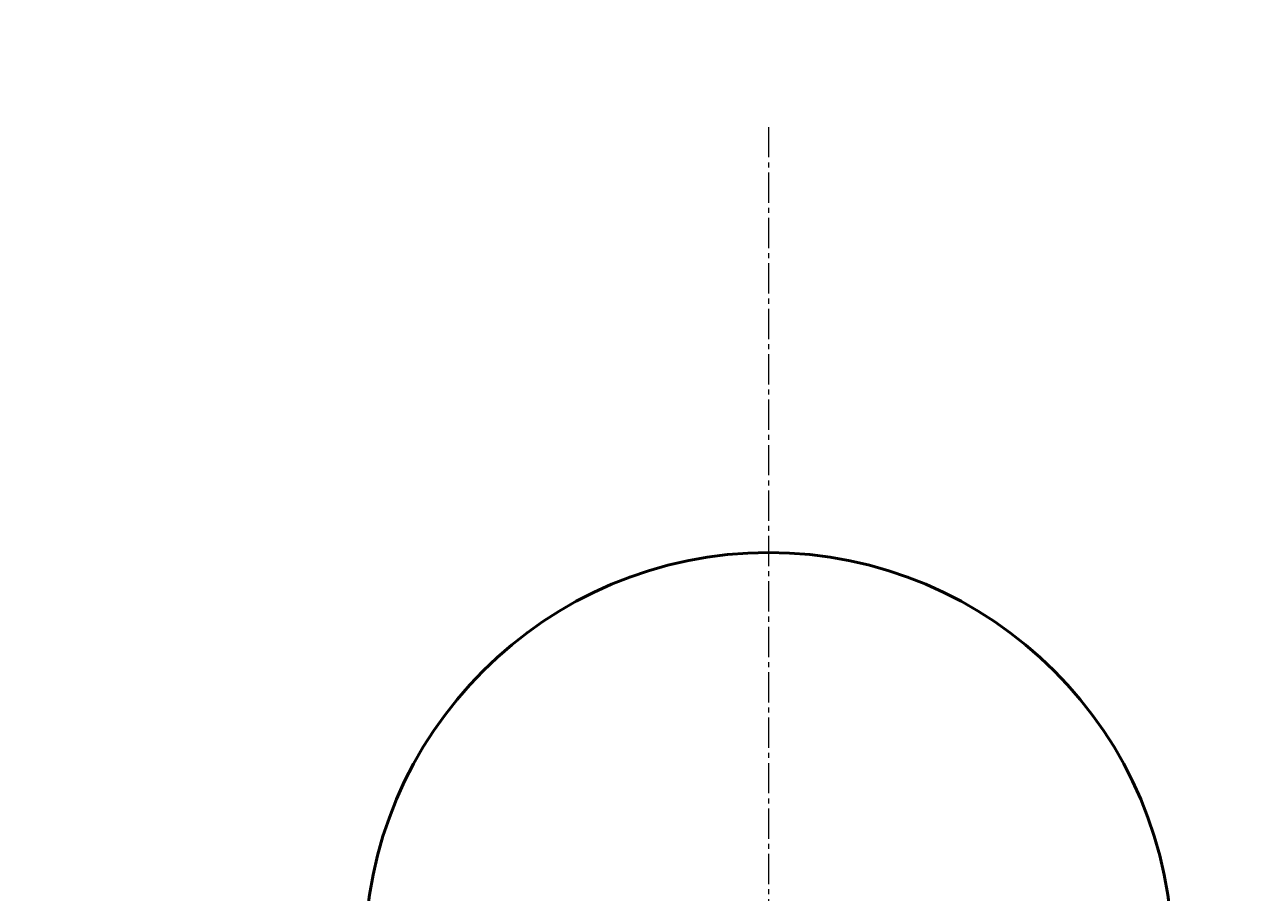
# Model space of a CAD drawing. Units: millimetres. Extents: x -60 to 113, y -37 to 126.
# Tile 11 of 17: x 19 to 49, y 48 to 70. Entities that reach past the tile are written whole.
import ezdxf

# ---------------------------------------------------------------- set-up
doc = ezdxf.new("R2010")
doc.units = ezdxf.units.MM
doc.header["$MEASUREMENT"] = 0
doc.linetypes.add('CENTER2', pattern=[1.125, 0.75, -0.125, 0.125, -0.125])
for name, color, linetype, lineweight in [('M-CNTR', 4, 'CENTER2', 18), ('M-DIMS', 2, 'Continuous', 25), ('M-OUTL', 7, 'Continuous', 50)]:
    doc.layers.add(name, color=color, linetype=linetype, lineweight=lineweight)
doc.styles.get("Standard").update_dxf_attribs({"font": 'arial.ttf'})
doc.dimstyles.get("Standard").update_dxf_attribs({"dimtxt": 0.18, "dimasz": 0.18, "dimexe": 0.18, "dimexo": 0.0625, "dimgap": 0.09, "dimtad": 0, "dimtih": 1, "dimtoh": 1, "dimdec": 4, "dimzin": 0, "dimdsep": 46, "dimtxsty": 'Standard', "dimcen": 0.09, "dimadec": 0, "dimazin": 0, "dimtfac": 1, "dimtdec": 4, "dimtofl": 0, "dimtmove": 0, "dimatfit": 3, "dimfxl": 1, "dimtolj": 1, "dimtzin": 0, "dimarcsym": 0})

# ---------------------------------------------------------------- blocks, each defined once
blk = doc.blocks.new('*D7')
at = {"layer": 'Defpoints', "color": 0, "transparency": 16777216}
for p in [(48.606, 76.822), (-30.775, 49.351)]:
    blk.add_point(p, dxfattribs=at)
at = {"layer": 'M-DIMS', "color": 0, "lineweight": -2, "transparency": 16777216}
for p, q in [((37.821, 73.09), (48.435, 76.764)), ((37.641, 73.09), (37.821, 73.09))]:
    blk.add_line(p, q, dxfattribs=at)
at = {"layer": 'M-DIMS', "color": 0, "transparency": 16777216}
blk.add_solid([(48.426, 76.792), (48.445, 76.735), (48.606, 76.822)], dxfattribs=at)
at = {"layer": 'M-DIMS', "color": 0, "transparency": 16777216, "insert": (35.165, 73.09), "char_height": 0.18, "attachment_point": 5}
blk.add_mtext('\\A1;{\\H11.11111x;R84}', dxfattribs=at)
blk = doc.blocks.new('*D11')
at = {"layer": 'Defpoints', "color": 0, "transparency": 16777216}
for p in [(32.38, 55.737), (41.75, 38.068)]:
    blk.add_point(p, dxfattribs=at)
at = {"layer": 'M-DIMS', "color": 0, "lineweight": -2, "transparency": 16777216}
for p, q in [((37.065, 46.813), (37.065, 46.993)), ((36.975, 46.903), (37.155, 46.903)), ((46.107, 29.851), (41.834, 37.909)), ((46.287, 29.851), (46.107, 29.851))]:
    blk.add_line(p, q, dxfattribs=at)
at = {"layer": 'M-DIMS', "color": 0, "transparency": 16777216}
blk.add_solid([(41.861, 37.923), (41.808, 37.895), (41.75, 38.068)], dxfattribs=at)
at = {"layer": 'M-DIMS', "color": 0, "transparency": 16777216, "insert": (48.894, 29.851), "char_height": 0.18, "attachment_point": 5}
blk.add_mtext('\\A1;{\\H11.11111x;%%C20}', dxfattribs=at)
blk = doc.blocks.new('*D17')
at = {"layer": 'Defpoints', "color": 0, "transparency": 16777216}
for p in [(67.355, 124.823), (10.532, 88.533), (67.355, 6.442)]:
    blk.add_point(p, dxfattribs=at)
at = {"layer": 'M-DIMS', "color": 0, "lineweight": -2, "transparency": 16777216}
for p, q in [((10.532, 88.595), (10.532, 125.003)), ((10.712, 124.823), (37.422, 124.823)), ((67.175, 124.823), (40.465, 124.823)), ((67.355, 6.504), (67.355, 125.003))]:
    blk.add_line(p, q, dxfattribs=at)
at = {"layer": 'M-DIMS', "color": 0, "transparency": 16777216}
for points in [[(10.712, 124.853), (10.712, 124.793), (10.532, 124.823)], [(67.175, 124.853), (67.175, 124.793), (67.355, 124.823)]]:
    blk.add_solid(points, dxfattribs=at)
at = {"layer": 'M-DIMS', "color": 0, "transparency": 16777216, "insert": (38.944, 124.823), "char_height": 0.18, "attachment_point": 5}
blk.add_mtext('\\A1;{\\H11.11111x;56}', dxfattribs=at)
blk = doc.blocks.new('*D23')
at = {"layer": 'Defpoints', "color": 0, "transparency": 16777216}
for p in [(44.117, 53.993), (30.013, 39.813)]:
    blk.add_point(p, dxfattribs=at)
at = {"layer": 'M-DIMS', "color": 0, "lineweight": -2, "transparency": 16777216}
for p, q in [((37.065, 46.813), (37.065, 46.993)), ((36.975, 46.903), (37.155, 46.903)), ((25.781, 35.559), (29.886, 39.685)), ((25.601, 35.559), (25.781, 35.559))]:
    blk.add_line(p, q, dxfattribs=at)
at = {"layer": 'M-DIMS', "color": 0, "transparency": 16777216}
blk.add_solid([(29.864, 39.706), (29.907, 39.664), (30.013, 39.813)], dxfattribs=at)
at = {"layer": 'M-DIMS', "color": 0, "transparency": 16777216, "insert": (24.97, 35.559), "char_height": 0.18, "attachment_point": 5}
blk.add_mtext('\\A1;∅20.0000', dxfattribs=at)
blk = doc.blocks.new('*D24')
at = {"layer": 'Defpoints', "color": 0, "transparency": 16777216}
for p in [(48.596, 76.851), (-30.775, 49.351)]:
    blk.add_point(p, dxfattribs=at)
at = {"layer": 'M-DIMS', "color": 0, "lineweight": -2, "transparency": 16777216}
for p, q in [((96.218, 93.35), (48.766, 76.909)), ((96.398, 93.35), (96.218, 93.35)), ((-30.775, 49.261), (-30.775, 49.441)), ((-30.865, 49.351), (-30.685, 49.351))]:
    blk.add_line(p, q, dxfattribs=at)
at = {"layer": 'M-DIMS', "color": 0, "transparency": 16777216}
blk.add_solid([(48.756, 76.938), (48.776, 76.881), (48.596, 76.851)], dxfattribs=at)
at = {"layer": 'M-DIMS', "color": 0, "transparency": 16777216, "insert": (97.018, 93.35), "char_height": 0.18, "attachment_point": 5}
blk.add_mtext('\\A1;R84.0000', dxfattribs=at)

msp = doc.modelspace()

# ---------------------------------------------------------------- linework, layer by layer
at = {"layer": 'M-CNTR'}
msp.add_line((37.06129, 67.44095), (37.06756, 28.90573), dxfattribs=at)
at = {"layer": 'M-OUTL'}
msp.add_circle((37.06463, 46.90263), 10, dxfattribs=at)
msp.add_arc((-30.77517, 49.3506), 84, 356.2470441, 43.4253235, dxfattribs=at)

# ---------------------------------------------------------------- dimensions: what is measured, and where the dimension line sits
at = {"layer": 'M-DIMS'}
dim = msp.add_linear_dim(base=(67.35481, 124.82251), p1=(10.53227, 88.53289), p2=(67.35481, 6.44179), text='{\\H11.11111x;56}', dimstyle='Standard', override={"dimclrd": 0, "dimclre": 0, "dimclrt": 0}, dxfattribs=at)
dim.commit()
dim.dimension.update_dxf_attribs({"geometry": '*D17', "text_midpoint": (38.94354, 124.82251)})
dim = msp.add_radius_dim(center=(-30.77517, 49.3506), mpoint=(48.59582, 76.85052), dimstyle='Standard', override={"dimdec": 4, "dimlfac": 1, "dimrnd": 0, "dimzin": 0, "dimdsep": 46, "dimlunit": 2}, dxfattribs=at)
dim.commit()
dim.dimension.update_dxf_attribs({"geometry": '*D24', "text_midpoint": (97.01779, 93.35047), "dimtype": 164})
dim = msp.add_radius_dim(center=(-30.77517, 49.3506), mpoint=(48.60556, 76.82239), text='{\\H11.11111x;R84}', dimstyle='Standard', override={"dimclrd": 0, "dimclre": 0, "dimclrt": 0}, dxfattribs=at)
dim.commit()
dim.dimension.update_dxf_attribs({"geometry": '*D7', "text_midpoint": (35.16548, 73.09007), "dimtype": 164})
dim = msp.add_diameter_dim_2p(p1=(32.37959, 55.73724), p2=(41.74967, 38.06802), text='{\\H11.11111x;%%C20}', dimstyle='Standard', override={"dimclrd": 0, "dimclre": 0, "dimclrt": 0}, dxfattribs=at)
dim.commit()
dim.dimension.update_dxf_attribs({"geometry": '*D11', "text_midpoint": (48.8944, 29.85072), "dimtype": 163})
dim = msp.add_diameter_dim_2p(p1=(44.11671, 53.99263), p2=(30.01255, 39.81262), dimstyle='Standard', override={"dimdec": 4, "dimlfac": 1, "dimrnd": 0, "dimzin": 0, "dimdsep": 46, "dimlunit": 2}, dxfattribs=at)
dim.commit()
dim.dimension.update_dxf_attribs({"geometry": '*D23', "text_midpoint": (24.97014, 35.55862), "dimtype": 163})

doc.saveas('drawing.dxf')
